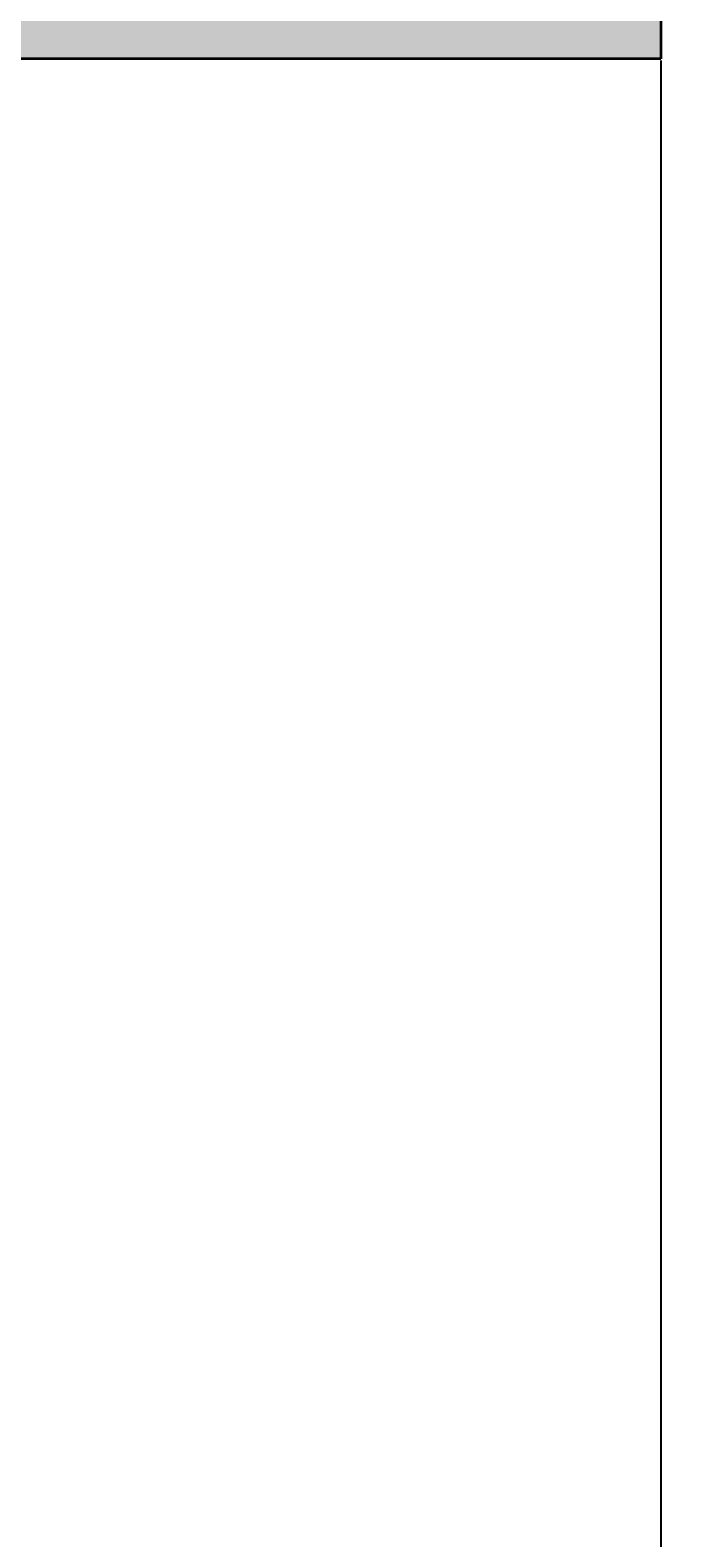
# Model space of a CAD drawing. Units: inches. Extents: x 1998 to 2588, y 1139 to 1977.
# Tile 111 of 134: x 2528 to 2550, y 1427 to 1477. Entities that reach past the tile are written whole.
import ezdxf

# ---------------------------------------------------------------- set-up
doc = ezdxf.new("R2010")
doc.units = ezdxf.units.IN
for name, color, linetype, lineweight in [('A-ANNO-DIMS', 2, 'Continuous', 18), ('A-WALL-PATT', 252, 'Continuous', 13), ('WALL', 200, 'Continuous', 35)]:
    doc.layers.add(name, color=color, linetype=linetype, lineweight=lineweight)
doc.styles.get("Standard").update_dxf_attribs({"font": 'arial.ttf'})
doc.dimstyles.get("Standard").update_dxf_attribs({"dimtxt": 0.18, "dimasz": 0.18, "dimexe": 0.18, "dimexo": 0.0625, "dimgap": 0.09, "dimtad": 0, "dimtih": 1, "dimtoh": 1, "dimdec": 4, "dimzin": 0, "dimdsep": 46, "dimtxsty": 'Standard', "dimcen": 0.09, "dimadec": 0, "dimazin": 0, "dimtfac": 1, "dimtdec": 4, "dimtofl": 0, "dimtmove": 0, "dimatfit": 3, "dimfxl": 1, "dimtolj": 1, "dimtzin": 0, "dimarcsym": 0})

# ---------------------------------------------------------------- blocks, each defined once
blk = doc.blocks.new('*D23')
at = {"layer": 'A-ANNO-DIMS', "color": 0, "lineweight": -2, "transparency": 16777216}
for p, q in [((2549.179, 1476.17), (2549.179, 1138.602)), ((2059.473, 1413.17), (2059.473, 1138.602)), ((2059.653, 1138.782), (2303.928, 1138.782)), ((2548.999, 1138.782), (2304.723, 1138.782))]:
    blk.add_line(p, q, dxfattribs=at)
at = {"layer": 'A-ANNO-DIMS', "color": 0, "transparency": 16777216}
for points in [[(2059.653, 1138.812), (2059.653, 1138.752), (2059.473, 1138.782)], [(2548.999, 1138.812), (2548.999, 1138.752), (2549.179, 1138.782)]]:
    blk.add_solid(points, dxfattribs=at)
at = {"layer": 'Defpoints', "color": 0, "transparency": 16777216}
for p in [(2549.179, 1476.232), (2059.473, 1413.232), (2549.179, 1138.782)]:
    blk.add_point(p, dxfattribs=at)
at = {"layer": 'A-ANNO-DIMS', "color": 0, "transparency": 16777216, "insert": (2304.326, 1138.782), "char_height": 0.18, "attachment_point": 5}
blk.add_mtext('\\A1;489.7', dxfattribs=at)
blk = doc.blocks.new('*D24')
at = {"layer": 'A-ANNO-DIMS', "color": 0, "lineweight": -2, "transparency": 16777216}
for p, q in [((2398.535, 1911.232), (2588.309, 1911.232)), ((2588.129, 1911.052), (2588.129, 1570.164)), ((2588.129, 1228.912), (2588.129, 1569.8)), ((2527.535, 1228.732), (2588.309, 1228.732))]:
    blk.add_line(p, q, dxfattribs=at)
at = {"layer": 'A-ANNO-DIMS', "color": 0, "transparency": 16777216}
for points in [[(2588.099, 1911.052), (2588.159, 1911.052), (2588.129, 1911.232)], [(2588.099, 1228.912), (2588.159, 1228.912), (2588.129, 1228.732)]]:
    blk.add_solid(points, dxfattribs=at)
at = {"layer": 'Defpoints', "color": 0, "transparency": 16777216}
for p in [(2398.473, 1911.232), (2588.129, 1911.232), (2527.473, 1228.732)]:
    blk.add_point(p, dxfattribs=at)
at = {"layer": 'A-ANNO-DIMS', "color": 0, "transparency": 16777216, "insert": (2588.129, 1569.982), "char_height": 0.18, "attachment_point": 5}
blk.add_mtext('\\A1;682.5', dxfattribs=at)

msp = doc.modelspace()

# ---------------------------------------------------------------- hatches: boundary and pattern name
at = {"layer": 'A-WALL-PATT'}
h = msp.add_hatch(color=256, dxfattribs=at)
h.dxf.hatch_style = 1
h.paths.add_polyline_path([(2527.4729, 1362.2324), (2510.9729, 1362.2324), (2510.9729, 1357.7324), (2518.4729, 1357.7324), (2518.4729, 1237.7324), (2503.1458, 1237.7324), (2503.1458, 1228.7324), (2527.4729, 1228.7324)])
h.paths.add_polyline_path([(2490.5682, 1362.2324), (2398.4729, 1362.2324), (2398.4729, 1357.7324), (2490.5682, 1357.7324)])
h.paths.add_polyline_path([(2224.9729, 1264.7324), (2222.9729, 1264.7324), (2222.9729, 1232.4125), (2341.4729, 1232.4125), (2341.4729, 1234.4125), (2224.9729, 1234.4125)])
h.paths.add_polyline_path([(2334.5332, 1273.7324), (2264.7638, 1273.7324), (2264.7638, 1269.5611, -0.043659), (2264.3413, 1264.7324), (2334.5332, 1264.7324)])
h.paths.add_polyline_path([(2236.9551, 1273.7324), (2234.4125, 1273.7324), (2234.4125, 1264.7324), (2236.9551, 1264.7324), (2236.9551, 1269.5611)])
h.paths.add_polyline_path([(2222.9729, 1293.2324), (2096.9729, 1293.2324), (2096.9729, 1345.0966), (2087.9729, 1345.0966), (2087.9729, 1284.2324), (2222.9729, 1284.2324), (2222.9729, 1285.137)])
h.paths.add_polyline_path([(2096.9729, 1458.7927), (2087.9729, 1458.7927), (2087.9729, 1417.7324), (2087.9729, 1413.2324), (2096.9729, 1413.2324), (2096.9729, 1417.7324)])
h.paths.add_polyline_path([(2096.9729, 1413.2324), (2087.9729, 1413.2324), (2087.9729, 1365.5012), (2096.9729, 1365.5012), (2096.9729, 1369.3358)])
h.paths.add_polyline_path([(2186.2943, 1417.7324), (2138.6074, 1417.7324), (2096.9729, 1417.7324), (2096.9729, 1413.2324), (2138.6074, 1413.2324), (2186.2943, 1413.2324)])
h.paths.add_polyline_path([(2181.4729, 1465.7324), (2176.9729, 1465.7324), (2176.9729, 1451.6434), (2181.4729, 1451.6434)])
h.paths.add_polyline_path([(2181.4729, 1422.1664), (2176.9729, 1422.1664), (2176.9729, 1417.7324), (2181.4729, 1417.7324)])
h.paths.add_polyline_path([(2063.9729, 1465.7324), (2087.9729, 1465.7324), (2087.9729, 1470.2324), (2059.4729, 1470.2324), (2059.4729, 1413.2324), (2087.9729, 1413.2324), (2087.9729, 1417.7324), (2063.9729, 1417.7324)])
h.paths.add_polyline_path([(2181.4729, 1755.2324), (2176.9729, 1755.2324), (2176.9729, 1748.6798), (2177.0513, 1748.6798), (2181.4729, 1748.6798)])
h.paths.add_polyline_path([(2227.4729, 1707.2324), (2220.4647, 1707.2324), (2220.4647, 1702.7324), (2222.9729, 1702.7324), (2222.9729, 1604.637), (2227.4729, 1604.637)])
h.paths.add_polyline_path([(2114.9729, 1702.7324), (2105.9729, 1702.7324), (2105.9729, 1628.4781, -0.0318759), (2110.1012, 1628.7416), (2114.9729, 1628.7416)])
h.paths.add_polyline_path([(2345.9729, 1739.3278), (2341.4729, 1739.3278), (2341.4729, 1647.5211), (2345.9729, 1647.5211)])
h.paths.add_polyline_path([(2350.6273, 1641.2324), (2345.9729, 1641.2324), (2345.9729, 1636.7324), (2350.6273, 1636.7324), (2350.6273, 1639.8729)])
h.paths.add_polyline_path([(2501.9729, 1641.2324), (2407.9729, 1641.2324), (2392.5005, 1641.2324), (2392.5005, 1639.8729), (2392.5005, 1636.7324), (2501.9729, 1636.7324)])
h.paths.add_polyline_path([(2510.9729, 1755.2324), (2501.9729, 1755.2324), (2501.9729, 1641.2324), (2510.9729, 1641.2324)])
h.paths.add_polyline_path([(2549.1786, 1641.2324), (2522.3775, 1641.2324), (2522.3775, 1636.7324), (2540.1786, 1636.7324), (2540.1786, 1480.7324), (2522.3775, 1480.7324), (2522.3775, 1476.2324), (2549.1786, 1476.2324)])
h.paths.add_polyline_path([(2498.1786, 1594.7324), (2407.9729, 1594.7324), (2407.9729, 1585.7324), (2416.9729, 1585.7324), (2489.1786, 1585.7324), (2489.1786, 1531.7324), (2416.9729, 1531.7324), (2407.9729, 1531.7324), (2407.9729, 1522.7324), (2498.1786, 1522.7324)])
h.paths.add_polyline_path([(2351.6437, 1480.7324), (2345.9729, 1480.7324), (2345.9729, 1476.2324), (2351.6437, 1476.2324), (2351.6437, 1477.5919)])
h.paths.add_polyline_path([(2501.9729, 1480.7324), (2498.1786, 1480.7324), (2407.9729, 1480.7324), (2393.5168, 1480.7324), (2393.5168, 1477.5919), (2393.5168, 1476.2324), (2501.9729, 1476.2324)])

# ---------------------------------------------------------------- linework, layer by layer
at = {"layer": 'WALL'}
for p, q in [((2549.1786, 1641.2324), (2549.1786, 1476.2324)), ((2549.1786, 1476.2324), (2522.3775, 1476.2324))]:
    msp.add_line(p, q, dxfattribs=at)

# ---------------------------------------------------------------- dimensions: what is measured, and where the dimension line sits
at = {"layer": 'A-ANNO-DIMS'}
dim = msp.add_linear_dim(base=(2588.1286, 1911.2324), p1=(2527.4729, 1228.7324), p2=(2398.4729, 1911.2324), angle=90, dimstyle='Standard', override={"dimdec": 1, "dimlfac": 1, "dimrnd": 0, "dimzin": 0, "dimdsep": 46, "dimlunit": 2}, dxfattribs=at)
dim.commit()
dim.dimension.update_dxf_attribs({"geometry": '*D24', "text_midpoint": (2588.1286, 1569.9824)})
dim = msp.add_linear_dim(base=(2549.1786, 1138.7824), p1=(2059.4729, 1413.2324), p2=(2549.1786, 1476.2324), dimstyle='Standard', override={"dimdec": 1, "dimlfac": 1, "dimrnd": 0, "dimzin": 0, "dimdsep": 46, "dimlunit": 2}, dxfattribs=at)
dim.commit()
dim.dimension.update_dxf_attribs({"geometry": '*D23', "text_midpoint": (2304.3257, 1138.7824)})

doc.saveas('drawing.dxf')
